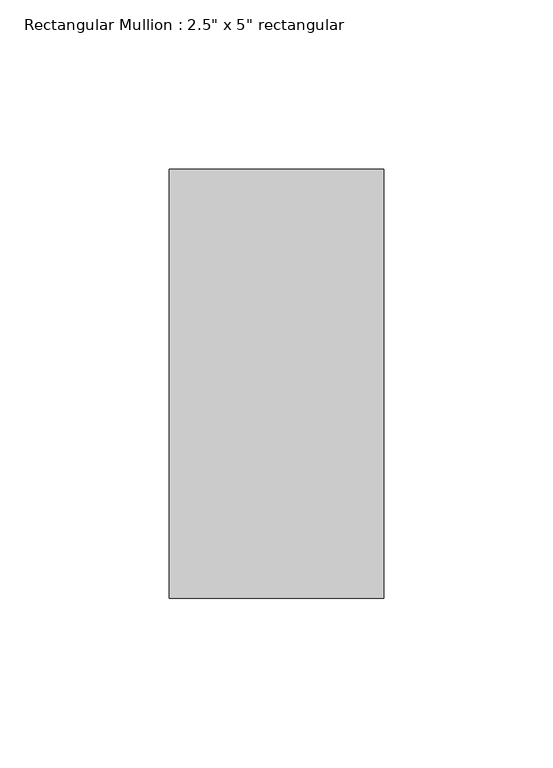
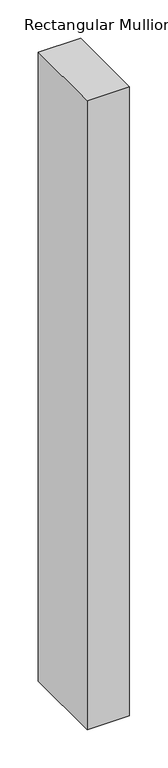
"""IFC4 building model written with IfcOpenShell, lengths in millimetres: member geometry."""

from ifc_helpers import new_model, si_unit, frame, origin, place, context, project, spatial, polyline, outline, extrude, source, transform, mapped, element, save


def member_948b814d(model_context):
    return source(origin(), model_context, "Body", "SweptSolid", [
        extrude(outline(polyline([(31.75, 63.5), (31.75, -63.5), (-31.75, -63.5), (-31.75, 63.5), (31.75, 63.5)])), frame((0.0, 0.0, -1001.0022263), z_axis=(0.0, 0.0, 1.0), x_axis=(1.0, 0.0, 0.0)), (0.0, 0.0, 1.0), 1001.0022263),
    ])


if __name__ == "__main__":
    model = new_model("IFC4")
    model_context = context("Model", 3, world=origin())
    ifc_project = project(units=[si_unit("LENGTHUNIT", "METRE", prefix="MILLI")], contexts=[model_context])
    site = spatial("IfcSite", under=ifc_project)
    building = spatial("IfcBuilding", under=site)
    placement = place(None, origin())
    member_shape = member_948b814d(model_context)
    element("IfcMember", 1, ObjectType="Rectangular Mullion : 2.5\" x 5\" rectangular", at=placement, inside=building, context=model_context, shape_type="MappedRepresentation", body=[
        mapped(member_shape, transform((0.0, 0.0, 0.0), x_axis=(1.0, 0.0, 0.0), y_axis=(0.0, 1.0, 0.0), z_axis=(0.0, 0.0, 1.0))),
    ])
    save(model, "model.ifc")

# Revit data of these elements
# Type "Rectangular Mullion : 2.5\" x 5\" rectangular"
#   built-in parameter 1007304 = 0.416667 (stored number, unit not read)
#   built-in parameter 1007301 = 0.104167 (stored number, unit not read)
#   built-in parameter 1007300 = 0.104167 (stored number, unit not read)
# Element 1 (IfcMember, "Rectangular Mullion : 2.5\" x 5\" rectangular")
#   Materials on its faces: "Aluminum"
# Materials
#   "Aluminum": class "Metal", colour RGB 247 247 247, transparency 0, Description = "Aluminum 6061", Cost = 0
